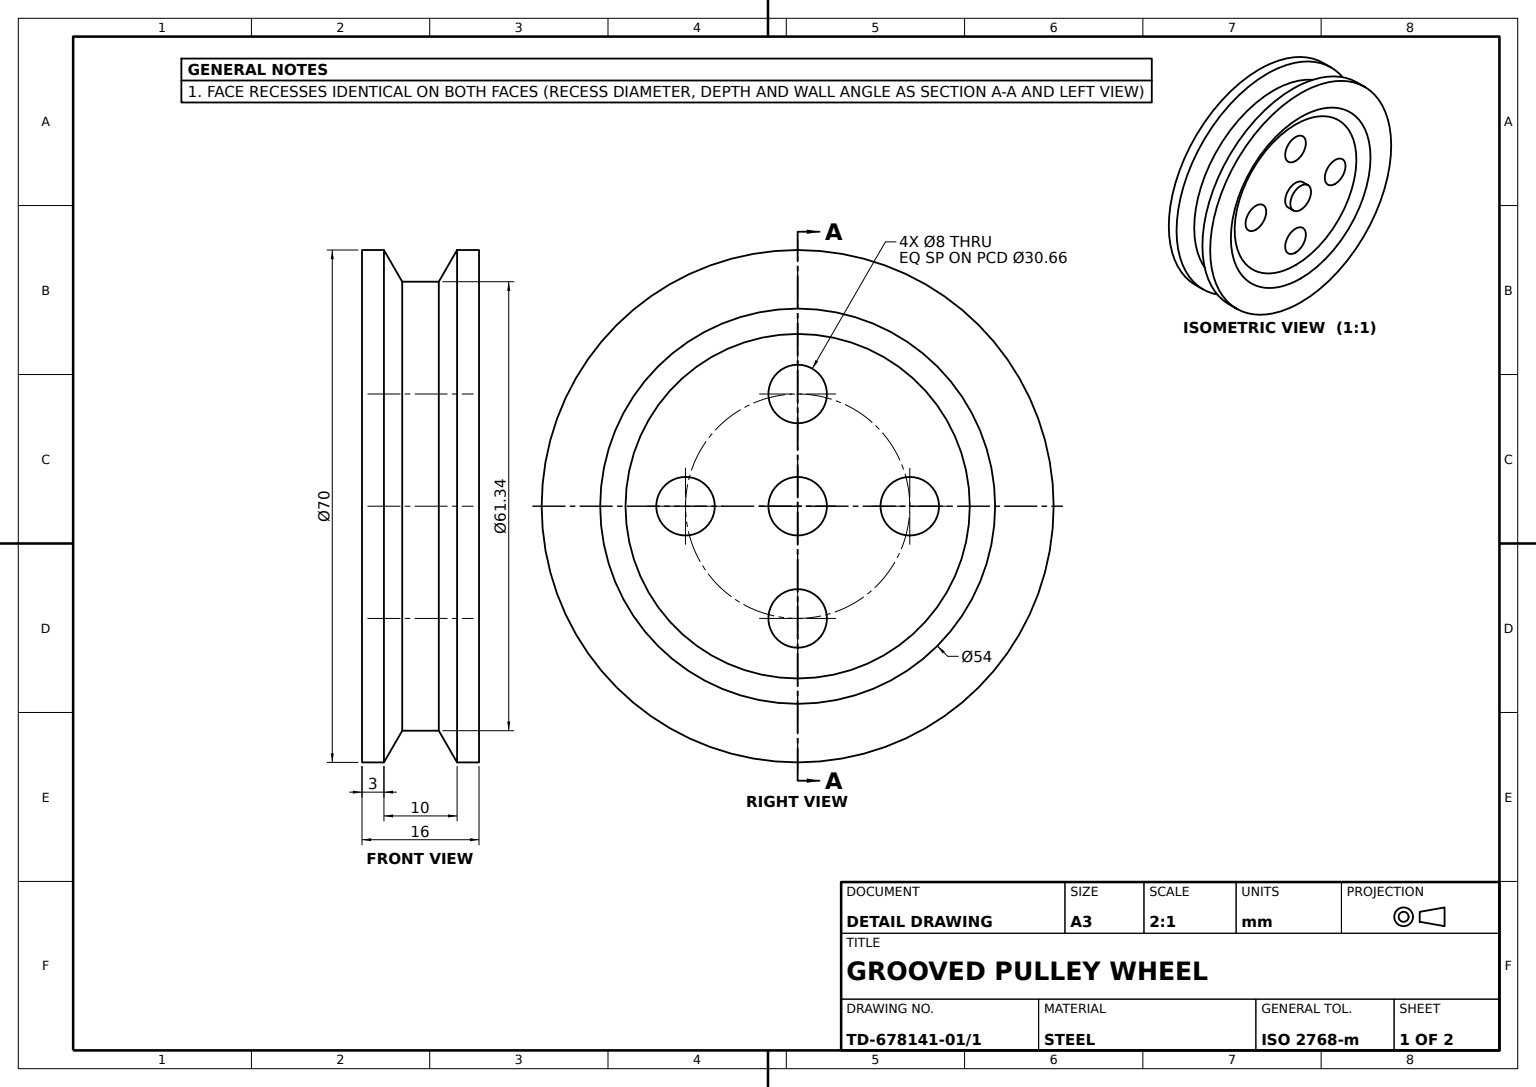
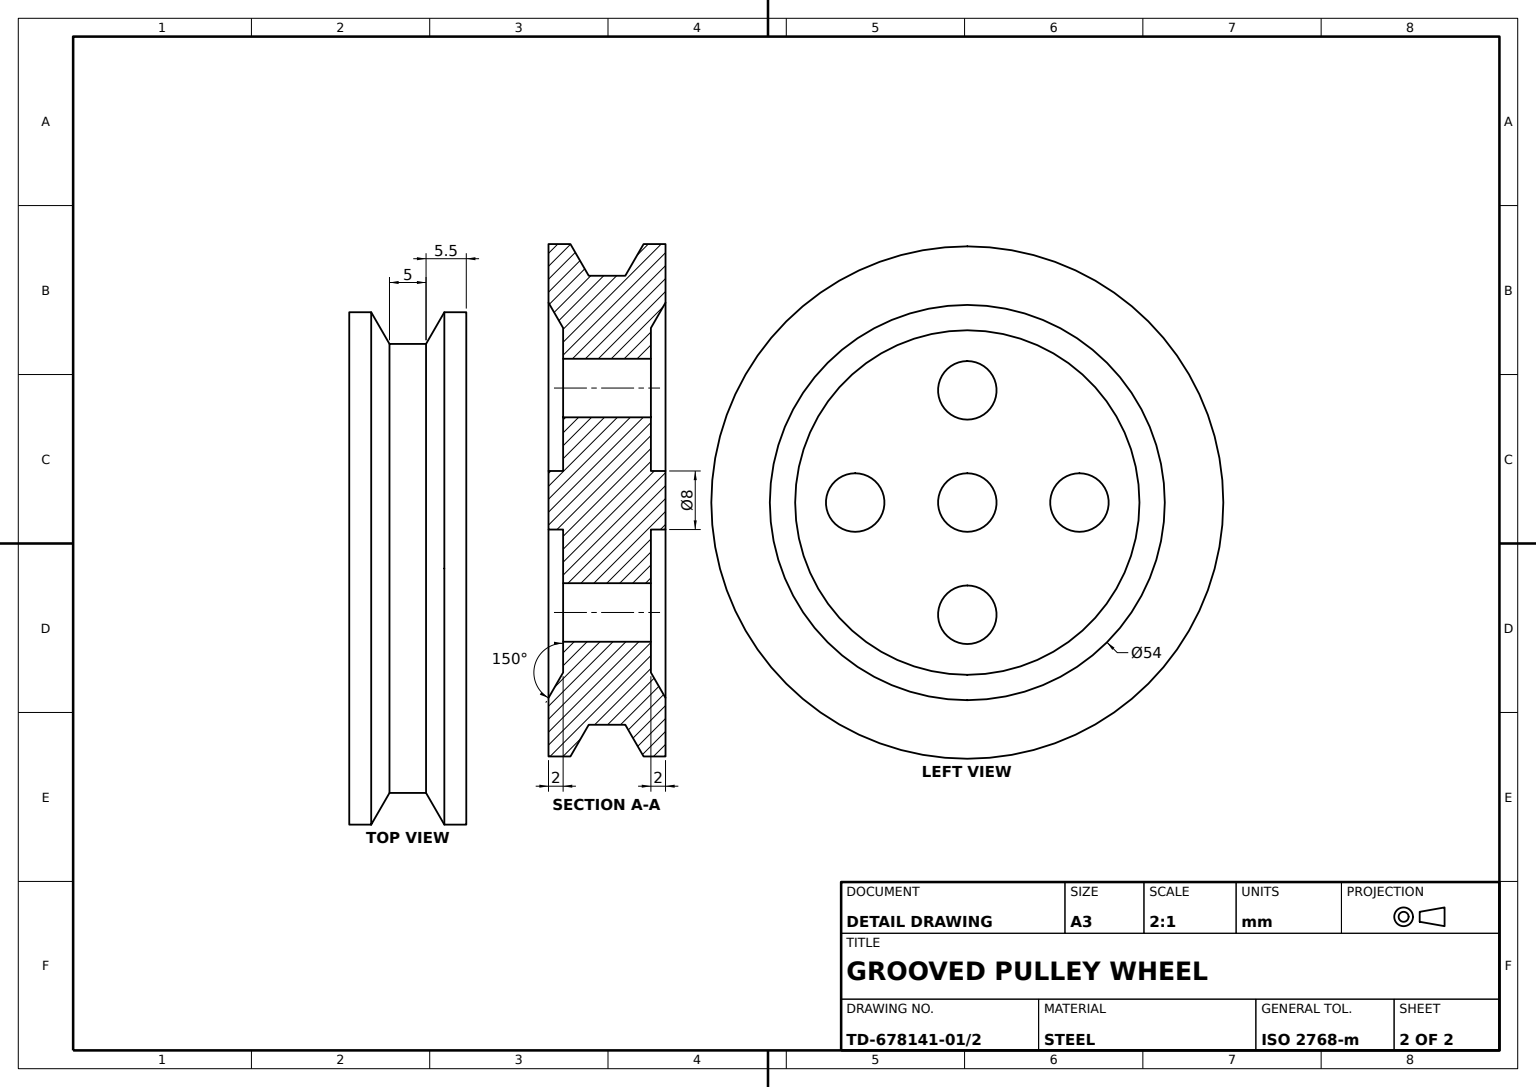
from build123d import *

# Parameters (mm, degrees)
HUB_HOLES_SKETCH_R = 4
HUB_HOLES_8_DEPTH  = 56.695601263


with BuildPart() as part:
    # Pulley Profile Sketch → Pulley Body (revolve)
    with BuildSketch(Plane.XY):
        Polygon((8, 6), (-8, 6), (-8, 10), (-6, 10), (-6, 29.535898385), (-8, 33), (-8, 41), (-5, 41), (-2.5, 36.669872981), (2.5, 36.669872981), (5, 41), (8, 41), (8, 33), (6, 29.535898385), (6, 10), (8, 10), align=None)
    revolve(axis=Axis((8, 6, 0), (-1, 0, 0)))

    # Hub Holes Sketch → Hub Holes Ø8 (cut, through all)
    with BuildSketch(Plane.ZY.offset(6)):
        with Locations(Location((0, 21.329563784, 0), (0, 0, 270))):
            Circle(HUB_HOLES_SKETCH_R)
        with Locations(Location((-15.329563784, 6, 0), (0, 0, 270))):
            Circle(HUB_HOLES_SKETCH_R)
        with Locations(Location((15.329563784, 6, 0), (0, 0, 270))):
            Circle(HUB_HOLES_SKETCH_R)
        with Locations(Location((0, -9.329563784, 0), (0, 0, 270))):
            Circle(HUB_HOLES_SKETCH_R)
    extrude(amount=-HUB_HOLES_8_DEPTH, mode=Mode.SUBTRACT)


solid = part.part
